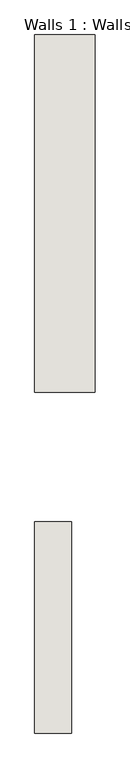
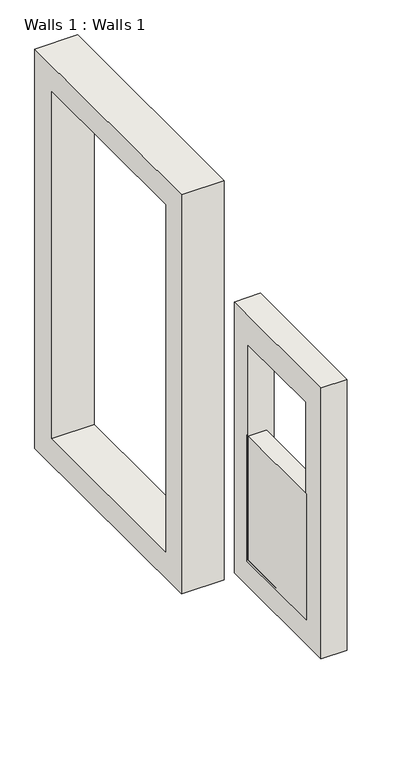
"""IFC4 building model written with IfcOpenShell, lengths in millimetres: wall geometry, Walls 1 : Walls 1."""

from ifc_helpers import new_model, si_unit, frame, origin, place, context, project, spatial, polyline, outline, extrude, source, transform, mapped, element, save


def walls_1_walls_1_5166138d(model_context):
    return source(origin(), model_context, "Body", "SweptSolid", [
        extrude(outline(polyline([(6368.6250851, 3910.4484418), (6368.6250851, 2207.5174218), (6063.8250851, 2207.5174218), (6063.8250851, 3910.4484418), (6368.6250851, 3910.4484418)])), frame((0.0, 0.0, 9341.7540643), z_axis=(0.0, 0.0, 1.0), x_axis=(1.0, 0.0, 0.0)), (0.0, 0.0, 1.0), 2212.535881),
        extrude(outline(polyline([(5803.3798743, 7620.0), (5803.3798743, 14630.4), (10019.7798743, 14630.4), (10019.7798743, 7620.0), (5803.3798743, 7620.0)]), holes=[polyline([(9539.8388399, 14175.0030784), (6263.2388399, 14175.0030784), (6263.2388399, 8079.0030784), (9539.8388399, 8079.0030784), (9539.8388399, 14175.0030784)])]), frame((6063.8250851, 0.0, 0.0), z_axis=(1.0, 0.0, 0.0), x_axis=(0.0, 1.0, 0.0)), (0.0, 0.0, 1.0), 711.2),
        extrude(outline(polyline([(1784.3255336, 8916.408286), (1784.3255336, 13670.8195407), (4279.3798743, 13670.8195407), (4279.3798743, 8916.408286), (1784.3255336, 8916.408286)]), holes=[polyline([(3881.6785739, 13148.1399453), (2239.2443881, 13148.1399453), (2239.2443881, 9380.7942683), (3881.6785739, 9380.7942683), (3881.6785739, 13148.1399453)])]), frame((6063.8250851, 0.0, 0.0), z_axis=(1.0, 0.0, 0.0), x_axis=(0.0, 1.0, 0.0)), (0.0, 0.0, 1.0), 431.9261591),
    ])


if __name__ == "__main__":
    model = new_model("IFC4")
    model_context = context("Model", 3, world=origin())
    ifc_project = project(units=[si_unit("LENGTHUNIT", "METRE", prefix="MILLI")], contexts=[model_context])
    site = spatial("IfcSite", under=ifc_project)
    building = spatial("IfcBuilding", under=site)
    placement = place(None, origin())
    walls_1_walls_1_shape = walls_1_walls_1_5166138d(model_context)
    element("IfcWall", 1, ObjectType="Walls 1 : Walls 1", at=placement, inside=building, context=model_context, shape_type="MappedRepresentation", body=[
        mapped(walls_1_walls_1_shape, transform((0.0, 0.0, 0.0), x_axis=(1.0, 0.0, 0.0), y_axis=(0.0, 1.0, 0.0), z_axis=(0.0, 0.0, 1.0))),
    ])
    save(model, "model.ifc")

# Revit data of these elements
# Element 1 (IfcWall, "Walls 1 : Walls 1")
#   Materials on its faces: "Default Wall"
# Materials
#   "Default Wall": colour RGB 128 128 128, transparency 0
